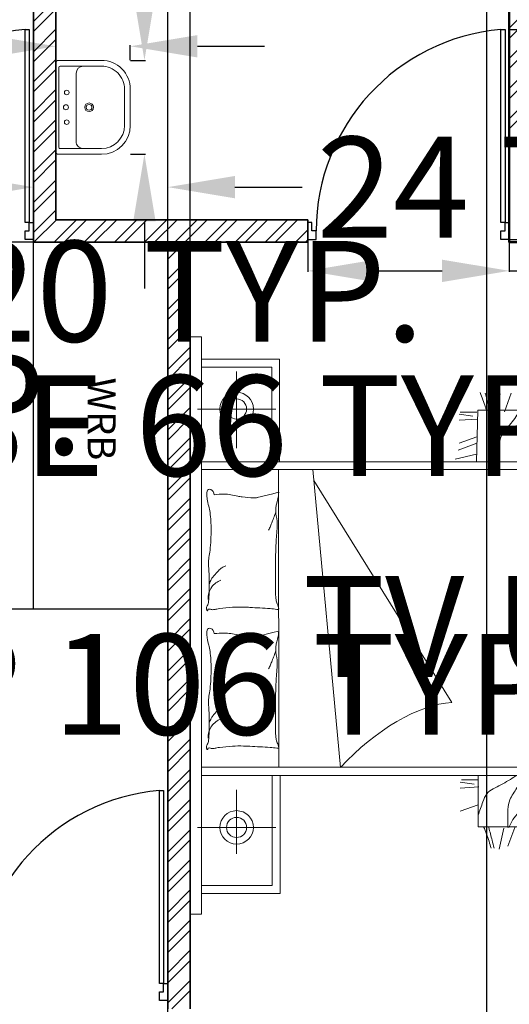
# Model space of a CAD drawing. Units: inches. Extents: x -90 to 536, y -553 to 299.
# Tile 23 of 27: x 207 to 294, y -2 to 174. Entities that reach past the tile are written whole.
import ezdxf

# ---------------------------------------------------------------- set-up
doc = ezdxf.new("R2010")
doc.units = ezdxf.units.IN
for name, color, linetype, lineweight in [('A-ANNO-DIMS', 2, 'Continuous', 18), ('A-ANNO-TEXT', 7, 'Continuous', 18), ('A-COLS', 7, 'Continuous', 50), ('A-DOOR', 4, 'Continuous', 25), ('A-FLOR-CASE', 2, 'Continuous', 25), ('A-FLOR-FIXT', 8, 'Continuous', 18), ('A-WALL-PATT', 252, 'Continuous', 13), ('Furniture', 2, 'Continuous', 18), ('Inner Wall', 5, 'Continuous', 35), ('Outer Wall', 1, 'Continuous', 50)]:
    doc.layers.add(name, color=color, linetype=linetype, lineweight=lineweight)
doc.styles.get("Standard").update_dxf_attribs({"font": 'arial.ttf'})
doc.dimstyles.get("Standard").update_dxf_attribs({"dimtxt": 18, "dimasz": 12, "dimexe": 0.18, "dimexo": 0.0625, "dimgap": 0.09, "dimtad": 0, "dimtih": 1, "dimtoh": 1, "dimdec": 0, "dimzin": 0, "dimdsep": 46, "dimlunit": 3, "dimtxsty": 'Standard', "dimcen": 0.09, "dimadec": 0, "dimazin": 0, "dimtfac": 1, "dimtdec": 0, "dimtofl": 0, "dimtmove": 0, "dimatfit": 3, "dimfxl": 1, "dimtolj": 1, "dimtzin": 0, "dimarcsym": 0})

# ---------------------------------------------------------------- blocks, each defined once
blk = doc.blocks.new('A$C57EA129C')
for p, q in [((0, 0.4428), (0, 0.1782)), ((0.016, 0.4589), (0.5631, 0.4589)), ((0.0356, 0.4321), (0.0356, 0.2896)), ((0.0445, 0.441), (0.5346, 0.441)), ((0.5435, 0.4321), (0.5435, 0.2896)), ((0.5791, 0.4428), (0.5791, 0.1782)), ((0.0802, 0.3341), (0.499, 0.3341)), ((0.0356, 0.2896), (0.0356, 0.1782)), ((0.5435, 0.2896), (0.5435, 0.1782)), ((0.1782, 0.0356), (0.4009, 0.0356)), ((0.1782, 0), (0.4009, 0))]:
    blk.add_line(p, q)
for centre, radius in [((0.1982, 0.392), 0.0143), ((0.2896, 0.3965), 0.0156), ((0.3809, 0.392), 0.0143), ((0.2896, 0.2545), 0.0267), ((0.2896, 0.2545), 0.0178)]:
    blk.add_circle(centre, radius)
for centre, radius, start, end in [((0.016, 0.4428), 0.016, 90, 180), ((0.0445, 0.4321), 0.00891, 90, 180), ((0.5346, 0.4321), 0.00891, 0, 90), ((0.5631, 0.4428), 0.016, 0, 90), ((0.0802, 0.2896), 0.0445, 90, 180), ((0.499, 0.2896), 0.0445, 0, 90), ((0.1782, 0.1782), 0.1782, 180, 270), ((0.1782, 0.1782), 0.1426, 180, 270), ((0.4009, 0.1782), 0.1782, 270, 0), ((0.4009, 0.1782), 0.1426, 270, 0)]:
    blk.add_arc(centre, radius, start, end)
blk = doc.blocks.new('A$C2B723114')
for p, q in [((0, 2.9047), (2.8274, 2.9047)), ((0, 2.8487), (0, 2.9047)), ((2.8274, 2.9047), (2.8274, 2.8487)), ((2.8274, 2.8487), (0, 2.8487)), ((0.1012, 2.4649), (0.1012, 2.849)), ((0.1396, 2.5033), (0.1396, 2.849)), ((0.4243, 2.8697), (0.4243, 2.4855)), ((0.6794, 0.7051), (0.6794, 2.8509)), ((0.7187, 0.7435), (0.7187, 2.8509)), ((2.1776, 2.8509), (2.1776, 0.7454)), ((2.216, 2.8509), (2.216, 0.707)), ((2.4742, 2.8697), (2.4742, 2.4855)), ((2.6798, 2.5052), (2.6798, 2.8509)), ((2.7182, 2.4668), (2.7182, 2.8509)), ((0.6087, 2.6776), (0.295, 2.6776)), ((2.6586, 2.6776), (2.2821, 2.6776)), ((1.3789, 2.4999), (1.3598, 2.5761)), ((2.0593, 2.4999), (2.0402, 2.5761)), ((0.6794, 2.4649), (0.1012, 2.4649)), ((0.6766, 2.5033), (0.1396, 2.5033)), ((0.7191, 2.47), (2.1778, 2.4719)), ((1.3858, 2.4723), (1.3789, 2.4999)), ((2.0662, 2.4723), (2.0593, 2.4999)), ((2.2188, 2.5052), (2.6798, 2.5052)), ((2.2188, 2.4668), (2.7182, 2.4668)), ((2.1771, 2.3036), (0.718, 2.1685)), ((1.0365, 1.6233), (2.1246, 2.2989)), ((2.2287, 1.6076), (2.2523, 1.5035)), ((2.2726, 1.593), (2.3061, 1.5007)), ((0.5047, 1.5819), (0.5353, 1.4945)), ((0.6174, 1.5819), (0.6232, 1.4916)), ((0.6467, 1.5819), (0.6369, 1.5137)), ((0.6571, 1.4945), (0.6571, 1.5765)), ((2.3067, 1.5881), (2.3373, 1.5007)), ((2.4194, 1.5881), (2.4251, 1.4979)), ((2.4487, 1.5881), (2.4389, 1.5199)), ((2.4591, 1.5007), (2.4591, 1.5828)), ((2.4685, 1.4964), (2.216, 1.5022)), ((2.4685, 1.4964), (2.4685, 0.0903)), ((0.4269, 0.0884), (0.4269, 1.4945)), ((0.4269, 1.4945), (0.6794, 1.4945)), ((2.4685, 1.4044), (2.5491, 1.3861)), ((0.3172, 1.3923), (0.4213, 1.3687)), ((2.4596, 1.3659), (2.552, 1.3324)), ((0.3318, 1.3485), (0.4241, 1.3149))]:
    blk.add_line(p, q)
for centre, radius in [((0.4243, 2.6776), 0.0821), ((2.4742, 2.6776), 0.0821), ((0.4243, 2.6776), 0.0493), ((2.4742, 2.6776), 0.0493)]:
    blk.add_circle(centre, radius)
for centre, radius, start, end in [((0.8078, 2.821), 0.00214, 160.436, 281.8931), ((0.8088, 2.8207), 0.00315, 111.7883, 160.436), ((0.8162, 2.8021), 0.0232, 94.3025, 111.7883), ((0.8091, 2.8151), 0.00394, 21.9904, 101.8931), ((0.8409, 2.7949), 0.0302, 158.579, 188.1335), ((0.7994, 2.8112), 0.0144, 338.579, 21.9904), ((0.8165, 2.7987), 0.0266, 59.3487, 94.3025), ((0.8554, 2.8643), 0.0497, 239.3487, 264.7408), ((0.9202, 3.5684), 0.7568, 264.7408, 268.0921), ((0.8679, 2.7254), 0.0915, 74.0648, 94.2159), ((0.8679, 2.7254), 0.0915, 53.9136, 74.0648), ((0.9409, 4.189), 1.3777, 268.0921, 270.5757), ((0.8679, 2.7254), 0.0915, 36.1766, 53.9136), ((0.86, 2.6097), 0.2158, 62.7604, 69.1397), ((0.9466, 3.6164), 0.8051, 270.5757, 274.8018), ((0.9263, 2.7386), 0.0708, 51.6114, 62.7604), ((1.0364, 2.548), 0.2671, 87.4614, 94.8018), ((1.042, 2.6745), 0.1405, 79.8101, 87.4614), ((1.1532, 3.2931), 0.488, 259.8101, 263.9133), ((1.204, 3.7695), 0.9671, 263.9133, 270), ((1.204, 3.4318), 0.6294, 270, 277.5469), ((1.2573, 3.0292), 0.2233, 277.5469, 285.744), ((1.3941, 2.5438), 0.281, 98.4372, 105.744), ((1.3747, 2.6748), 0.1486, 90, 98.4372), ((1.3713, 2.8186), 0.0315, 274.4002, 333.4195), ((1.3747, 2.74), 0.0833, 78.7276, 90), ((1.3886, 2.8099), 0.0121, 333.4195, 78.7276), ((1.4882, 2.821), 0.00214, 160.436, 281.8931), ((1.4892, 2.8207), 0.00315, 111.7883, 160.436), ((1.4966, 2.8021), 0.0232, 94.3025, 111.7883), ((1.4895, 2.8151), 0.00394, 21.9904, 101.8931), ((1.5213, 2.7949), 0.0302, 158.579, 188.1335), ((1.4798, 2.8112), 0.0144, 338.579, 21.9904), ((1.4969, 2.7987), 0.0266, 59.3487, 94.3025), ((1.5358, 2.8643), 0.0497, 239.3487, 264.7408), ((1.6006, 3.5684), 0.7568, 264.7408, 268.0921), ((1.5483, 2.7254), 0.0915, 74.0648, 94.2159), ((1.5483, 2.7254), 0.0915, 53.9136, 74.0648), ((1.6213, 4.189), 1.3777, 268.0921, 270.5757), ((1.5483, 2.7254), 0.0915, 36.1766, 53.9136), ((1.5404, 2.6097), 0.2158, 62.7604, 69.1397), ((1.627, 3.6164), 0.8051, 270.5757, 274.8018), ((1.6067, 2.7386), 0.0708, 51.6114, 62.7604), ((1.7168, 2.548), 0.2671, 87.4614, 94.8018), ((1.7224, 2.6745), 0.1405, 79.8101, 87.4614), ((1.8336, 3.2931), 0.488, 259.8101, 263.9133), ((1.8844, 3.7695), 0.9671, 263.9133, 270), ((1.8844, 3.4318), 0.6294, 270, 277.5469), ((1.9377, 3.0292), 0.2233, 277.5469, 285.744), ((2.0745, 2.5438), 0.281, 98.4372, 105.744), ((2.0551, 2.6748), 0.1486, 90, 98.4372), ((2.0517, 2.8186), 0.0315, 274.4002, 333.4195), ((2.0551, 2.74), 0.0833, 78.7276, 90), ((2.069, 2.8099), 0.0121, 333.4195, 78.7276), ((1.0356, 2.8227), 0.2268, 188.1335, 192.1095), ((0.635, 2.7368), 0.1829, 7.6809, 12.1095), ((-0.0181, 2.6487), 0.8418, 3.3687, 7.6809), ((0.8679, 2.7254), 0.0915, 18.4397, 36.1766), ((0.7461, 2.511), 0.3611, 46.1885, 51.6114), ((0.8523, 2.6218), 0.2076, 39.0349, 46.1885), ((0.9783, 2.7239), 0.0455, 28.3168, 39.0349), ((0.923, 2.7382), 0.4535, 0, 6.2324), ((1.716, 2.8227), 0.2268, 188.1335, 192.1095), ((1.3154, 2.7368), 0.1829, 7.6809, 12.1095), ((0.6623, 2.6487), 0.8418, 3.3687, 7.6809), ((1.5483, 2.7254), 0.0915, 18.4397, 36.1766), ((1.4265, 2.511), 0.3611, 46.1885, 51.6114), ((1.5327, 2.6218), 0.2076, 39.0349, 46.1885), ((1.6587, 2.7239), 0.0455, 28.3168, 39.0349), ((1.6034, 2.7382), 0.4535, 0, 6.2324), ((0.8558, 2.6579), 0.1846, 23.0028, 28.3168), ((0.5722, 2.8434), 0.8132, 347.8016, 350.3156), ((1.1884, 2.7382), 0.1881, 350.3156, 0), ((1.5362, 2.6579), 0.1846, 23.0028, 28.3168), ((1.2526, 2.8434), 0.8132, 347.8016, 350.3156), ((1.8688, 2.7382), 0.1881, 350.3156, 0), ((0.1976, 2.6614), 0.6258, 358.3669, 3.3687), ((1.6528, 2.6098), 0.2924, 167.8016, 171.9949), ((0.878, 2.6614), 0.6258, 358.3669, 3.3687), ((2.3332, 2.6098), 0.2924, 167.8016, 171.9949), ((-11.7321, 3.2823), 12.5718, 356.49514, 356.94504), ((-0.4351, 2.6794), 1.2587, 356.945, 358.3669), ((1.9648, 2.5659), 0.6074, 171.9949, 177.3351), ((-11.0517, 3.2823), 12.5718, 356.49514, 356.94504), ((0.2453, 2.6794), 1.2587, 356.945, 358.3669), ((2.6452, 2.5659), 0.6074, 171.9949, 177.3351), ((1.4204, 2.5912), 0.0624, 177.3351, 194.0452), ((2.1008, 2.5912), 0.0624, 177.3351, 194.0452), ((0.5206, 2.5319), 0.2961, 350.0016, 356.4951), ((1.4917, 3.1364), 0.681, 244.6889, 246.5156), ((1.4917, 3.1364), 0.681, 246.5156, 248.3423), ((1.201, 2.5319), 0.2961, 350.0016, 356.4951), ((2.1721, 3.1364), 0.681, 244.6889, 246.5156), ((2.1721, 3.1364), 0.681, 246.5156, 248.3423), ((0.8298, 2.4774), 0.0178, 170.0016, 196.6978), ((0.8139, 2.4726), 0.00122, 196.6978, 277.1204), ((0.8041, 2.5514), 0.0807, 277.1204, 286.2212), ((0.8068, 2.5419), 0.0707, 286.2212, 297.2841), ((0.8584, 2.4419), 0.0418, 102.869, 117.2841), ((0.879, 2.3515), 0.1345, 93.574, 102.869), ((0.9376, 1.4146), 1.0732, 90.2865, 93.574), ((0.9586, -2.7845), 5.2724, 89.0296, 90.2865), ((0.9954, -0.6123), 3.0999, 87.3904, 89.0296), ((1.0854, 1.364), 1.1216, 85.3824, 87.3904), ((1.28, 3.7729), 1.2952, 265.3824, 267.2509), ((1.228, 2.691), 0.2121, 267.2509, 281.5586), ((1.4917, 3.1364), 0.681, 248.3423, 250.572), ((1.4917, 3.1364), 0.681, 250.572, 252.8018), ((1.2975, 2.3514), 0.1345, 83.5659, 101.5586), ((1.3002, 2.3754), 0.1104, 72.6136, 83.5659), ((1.3965, 2.6828), 0.2118, 252.6136, 260.5159), ((1.4027, 2.7202), 0.2496, 260.5159, 265.9171), ((1.385, 2.4721), 0.000845, 265.9171, 14.0449), ((1.5102, 2.4774), 0.0178, 170.0016, 196.6978), ((1.4943, 2.4726), 0.00122, 196.6978, 277.1204), ((1.4845, 2.5514), 0.0807, 277.1204, 286.2212), ((1.4872, 2.5419), 0.0707, 286.2212, 297.2841), ((1.5388, 2.4419), 0.0418, 102.869, 117.2841), ((1.5594, 2.3515), 0.1345, 93.574, 102.869), ((1.618, 1.4146), 1.0732, 90.2865, 93.574), ((1.639, -2.7845), 5.2724, 89.0296, 90.2865), ((1.6758, -0.6123), 3.0999, 87.3904, 89.0296), ((1.7658, 1.364), 1.1216, 85.3824, 87.3904), ((1.9604, 3.7729), 1.2952, 265.3824, 267.2509), ((1.9084, 2.691), 0.2121, 267.2509, 281.5586), ((2.1721, 3.1364), 0.681, 248.3423, 250.572), ((2.1721, 3.1364), 0.681, 250.572, 252.8018), ((1.9779, 2.3514), 0.1345, 83.5659, 101.5586), ((1.9806, 2.3754), 0.1104, 72.6136, 83.5659), ((2.0769, 2.6828), 0.2118, 252.6136, 260.5159), ((2.0831, 2.7202), 0.2496, 260.5159, 265.9171), ((2.0654, 2.4721), 0.000845, 265.9171, 14.0449)]:
    blk.add_arc(centre, radius, start, end)
blk.add_ellipse((0.4962, 1.9132), major_axis=(0.4887, -0.4605), ratio=0.503305, start_param=0.491272, end_param=1.591113)
for points, knots in [([(0.427, 1.4678), (0.4036, 1.4582), (0.3693, 1.4441), (0.3335, 1.4344), (0.3221, 1.4313)], [0, 0, 0, 0, 98.452083, 144.639601, 144.639601, 144.639601, 144.639601]), ([(0.6768, 1.3104), (0.6615, 1.3339), (0.6315, 1.3797), (0.604, 1.4501), (0.5417, 1.4748), (0.5064, 1.4871), (0.4848, 1.4945)], [0, 0, 0, 0, 110.980521, 216.571322, 273.316778, 363.252298, 363.252298, 363.252298, 363.252298]), ([(2.5548, 1.4853), (2.5314, 1.4757), (2.5031, 1.4641), (2.4737, 1.4555), (2.4685, 1.454)], [0, 0, 0, 0, 98.452083, 119.481049, 119.481049, 119.481049, 119.481049]), ([(2.552, 1.4598), (2.5309, 1.4545), (2.5031, 1.4475), (2.4753, 1.4406), (2.4685, 1.4389)], [0, 0, 0, 0, 84.638756, 111.94623, 111.94623, 111.94623, 111.94623]), ([(0.4241, 1.4423), (0.4031, 1.437), (0.3691, 1.4284), (0.3351, 1.4199), (0.3221, 1.4167)], [0, 0, 0, 0, 84.638756, 136.955563, 136.955563, 136.955563, 136.955563]), ([(2.2145, 1.4211), (2.233, 1.4246), (2.2636, 1.4303), (2.2761, 1.3837), (2.3429, 1.3967), (2.3949, 1.3342), (2.4474, 1.3031), (2.4698, 1.2898)], [0, 0, 0, 0, 61.886907, 102.717887, 145.699352, 284.082577, 386.765171, 386.765171, 386.765171, 386.765171]), ([(0.6768, 1.286), (0.6567, 1.2911), (0.6145, 1.3017), (0.5543, 1.3533), (0.4816, 1.349), (0.4362, 1.3493), (0.4233, 1.3493)], [0, 0, 0, 0, 80.250278, 168.388677, 295.908361, 346.663112, 346.663112, 346.663112, 346.663112]), ([(0.4233, 1.3445), (0.4367, 1.3385), (0.464, 1.3264), (0.5129, 1.2848), (0.5456, 1.2161), (0.6131, 1.2349), (0.6142, 1.1913), (0.6642, 1.1806), (0.674, 1.144), (0.6817, 1.1154)], [0, 0, 0, 0, 56.745495, 115.23739, 254.956954, 286.678662, 337.828324, 366.201072, 468.500395, 468.500395, 468.500395, 468.500395])]:
    blk.add_open_spline(points, degree=3, knots=knots)
blk = doc.blocks.new('DOOR-36-A')
for points in [[(35.25, 37.5), (35.25, 3), (34.5, 3), (34.5, 37.5)], [(0, 0), (1.5, 0), (1.5, 1.5), (0.75, 1.5), (0.75, 3), (0, 3)], [(36, 0), (34.5, 0), (34.5, 1.5), (35.25, 1.5), (35.25, 3), (36, 3)]]:
    blk.add_lwpolyline(points, close=True)
blk.add_arc((37.64, 1.5), 36.14, 94.9791, 180)
blk = doc.blocks.new('COL-12X18')
blk.add_lwpolyline([(0, 18), (12, 18), (12, 0), (0, 0)], close=True)
blk = doc.blocks.new('WARDROBE')
blk.add_lwpolyline([(0, 65.56), (24, 65.56), (24, 0), (0, 0)], close=True)
blk = doc.blocks.new('*D19')
at = {"layer": 'A-ANNO-DIMS', "color": 0, "lineweight": -2, "transparency": 16777216}
for p, q in [((299.76, 172.45), (299.76, 184.45)), ((299.76, 184.45), (311.76, 184.45)), ((294.19, 172.45), (299.94, 172.45)), ((299.76, 146.95), (299.76, 160.45)), ((294.19, 134.95), (299.94, 134.95))]:
    blk.add_line(p, q, dxfattribs=at)
at = {"layer": 'A-ANNO-DIMS', "color": 0, "transparency": 16777216}
for points in [[(297.76, 160.45), (301.76, 160.45), (299.76, 172.45)], [(297.76, 146.95), (301.76, 146.95), (299.76, 134.95)]]:
    blk.add_solid(points, dxfattribs=at)
at = {"layer": 'Defpoints', "color": 0, "transparency": 16777216}
for p in [(294.13, 172.45), (299.76, 172.45), (294.13, 134.95)]:
    blk.add_point(p, dxfattribs=at)
at = {"layer": 'A-ANNO-DIMS', "color": 0, "transparency": 16777216, "insert": (408.3, 184.45), "char_height": 18, "attachment_point": 5}
blk.add_mtext('\\A1;DOOR A 38 TYP.', dxfattribs=at)
blk = doc.blocks.new('*D20')
at = {"layer": 'A-ANNO-DIMS', "color": 0, "lineweight": -2, "transparency": 16777216}
for p, q in [((258.13, 134.88), (258.13, 129.14)), ((294.13, 134.88), (294.13, 129.14)), ((270.13, 129.32), (282.13, 129.32)), ((294.13, 129.32), (306.13, 129.32))]:
    blk.add_line(p, q, dxfattribs=at)
at = {"layer": 'A-ANNO-DIMS', "color": 0, "transparency": 16777216}
for points in [[(270.13, 131.32), (270.13, 127.32), (258.13, 129.32)], [(282.13, 131.32), (282.13, 127.32), (294.13, 129.32)]]:
    blk.add_solid(points, dxfattribs=at)
at = {"layer": 'Defpoints', "color": 0, "transparency": 16777216}
for p in [(258.13, 134.95), (294.13, 134.95), (294.13, 129.32)]:
    blk.add_point(p, dxfattribs=at)
at = {"layer": 'A-ANNO-DIMS', "color": 0, "transparency": 16777216, "insert": (350.02, 129.32), "char_height": 18, "attachment_point": 5}
blk.add_mtext('\\A1;36 TYP.', dxfattribs=at)
blk = doc.blocks.new('*D25')
at = {"layer": 'A-ANNO-DIMS', "color": 0, "lineweight": -2, "transparency": 16777216}
for p, q in [((228.95, 178.94), (228.95, 190.94)), ((228.95, 190.94), (240.95, 190.94)), ((226.49, 166.94), (229.13, 166.94)), ((226.49, 150.15), (229.13, 150.15)), ((228.95, 138.15), (228.95, 126.15))]:
    blk.add_line(p, q, dxfattribs=at)
at = {"layer": 'A-ANNO-DIMS', "color": 0, "transparency": 16777216}
for points in [[(226.95, 178.94), (230.95, 178.94), (228.95, 166.94)], [(226.95, 138.15), (230.95, 138.15), (228.95, 150.15)]]:
    blk.add_solid(points, dxfattribs=at)
at = {"layer": 'Defpoints', "color": 0, "transparency": 16777216}
for p in [(226.43, 166.94), (228.95, 166.94), (226.43, 150.15)]:
    blk.add_point(p, dxfattribs=at)
at = {"layer": 'A-ANNO-DIMS', "color": 0, "transparency": 16777216, "insert": (325.67, 190.94), "char_height": 18, "attachment_point": 5}
blk.add_mtext('\\A1;BASIN 17 TYP.', dxfattribs=at)
blk = doc.blocks.new('*D26')
at = {"layer": 'A-ANNO-DIMS', "color": 0, "lineweight": -2, "transparency": 16777216}
for p, q in [((201.13, 169.45), (189.13, 169.45)), ((213.13, 167), (213.13, 169.63)), ((226.43, 167), (226.43, 169.63)), ((238.43, 169.45), (250.43, 169.45))]:
    blk.add_line(p, q, dxfattribs=at)
at = {"layer": 'A-ANNO-DIMS', "color": 0, "transparency": 16777216}
for points in [[(201.13, 171.45), (201.13, 167.45), (213.13, 169.45)], [(238.43, 171.45), (238.43, 167.45), (226.43, 169.45)]]:
    blk.add_solid(points, dxfattribs=at)
at = {"layer": 'Defpoints', "color": 0, "transparency": 16777216}
for p in [(213.13, 169.45), (213.13, 166.94), (226.43, 166.94)]:
    blk.add_point(p, dxfattribs=at)
at = {"layer": 'A-ANNO-DIMS', "color": 0, "transparency": 16777216, "insert": (146.08, 169.45), "char_height": 18, "attachment_point": 5}
blk.add_mtext('\\A1;13 TYP.', dxfattribs=at)
blk = doc.blocks.new('*D29')
at = {"layer": 'A-ANNO-DIMS', "color": 0, "lineweight": -2, "transparency": 16777216}
for p, q in [((357.07, 98.65), (347.09, 98.65)), ((347.27, 86.65), (347.27, 75.05)), ((347.27, 44.88), (347.27, 56.48)), ((357.07, 32.88), (347.09, 32.88))]:
    blk.add_line(p, q, dxfattribs=at)
at = {"layer": 'A-ANNO-DIMS', "color": 0, "transparency": 16777216}
for points in [[(345.27, 86.65), (349.27, 86.65), (347.27, 98.65)], [(345.27, 44.88), (349.27, 44.88), (347.27, 32.88)]]:
    blk.add_solid(points, dxfattribs=at)
at = {"layer": 'Defpoints', "color": 0, "transparency": 16777216}
for p in [(347.27, 98.65), (357.13, 98.65), (357.13, 32.88)]:
    blk.add_point(p, dxfattribs=at)
at = {"layer": 'A-ANNO-DIMS', "color": 0, "transparency": 16777216, "insert": (347.27, 65.76), "char_height": 18, "attachment_point": 5}
blk.add_mtext('\\A1;TV UNIT 66 TYP.', dxfattribs=at)
blk = doc.blocks.new('*D31')
at = {"layer": 'A-ANNO-DIMS', "color": 0, "lineweight": -2, "transparency": 16777216}
for p, q in [((90.45, 119.36), (100.65, 125.67)), ((100.65, 125.67), (112.65, 125.67)), ((78.67, 115.59), (80.34, 112.89)), ((61.33, 104.86), (63, 102.15)), ((52.7, 95.99), (42.5, 89.68))]:
    blk.add_line(p, q, dxfattribs=at)
at = {"layer": 'A-ANNO-DIMS', "color": 0, "transparency": 16777216}
for points in [[(89.4, 121.06), (91.5, 117.65), (80.24, 113.04)], [(51.65, 97.69), (53.76, 94.29), (62.91, 102.31)]]:
    blk.add_solid(points, dxfattribs=at)
at = {"layer": 'Defpoints', "color": 0, "transparency": 16777216}
for p in [(78.63, 115.64), (80.24, 113.04), (61.3, 104.91)]:
    blk.add_point(p, dxfattribs=at)
at = {"layer": 'A-ANNO-DIMS', "color": 0, "transparency": 16777216, "insert": (199.06, 125.67), "char_height": 18, "attachment_point": 5}
blk.add_mtext('\\A1;CHAIR 20 TYP.', dxfattribs=at)
blk = doc.blocks.new('*D33')
at = {"layer": 'A-ANNO-DIMS', "color": 0, "lineweight": -2, "transparency": 16777216}
for p, q in [((173.76, 108.4), (189.77, 108.4)), ((189.59, 96.4), (189.59, 64.83)), ((189.59, 14.45), (189.59, 46.02)), ((173.76, 2.45), (189.77, 2.45))]:
    blk.add_line(p, q, dxfattribs=at)
at = {"layer": 'A-ANNO-DIMS', "color": 0, "transparency": 16777216}
for points in [[(187.59, 96.4), (191.59, 96.4), (189.59, 108.4)], [(187.59, 14.45), (191.59, 14.45), (189.59, 2.45)]]:
    blk.add_solid(points, dxfattribs=at)
at = {"layer": 'Defpoints', "color": 0, "transparency": 16777216}
for p in [(173.7, 108.4), (173.7, 2.45), (189.59, 2.45)]:
    blk.add_point(p, dxfattribs=at)
at = {"layer": 'A-ANNO-DIMS', "color": 0, "transparency": 16777216, "insert": (189.59, 55.42), "char_height": 18, "attachment_point": 5}
blk.add_mtext('\\A1;BED GROUP 106 TYP.', dxfattribs=at)
blk = doc.blocks.new('*D37')
at = {"layer": 'A-ANNO-DIMS', "color": 0, "lineweight": -2, "transparency": 16777216}
for p, q in [((35.09, 103.75), (35.09, 105.68)), ((47.13, 103.75), (47.13, 105.68)), ((23.09, 105.5), (11.09, 105.5)), ((59.13, 105.5), (71.13, 105.5))]:
    blk.add_line(p, q, dxfattribs=at)
at = {"layer": 'A-ANNO-DIMS', "color": 0, "transparency": 16777216}
for points in [[(23.09, 107.5), (23.09, 103.5), (35.09, 105.5)], [(59.13, 107.5), (59.13, 103.5), (47.13, 105.5)]]:
    blk.add_solid(points, dxfattribs=at)
at = {"layer": 'Defpoints', "color": 0, "transparency": 16777216}
for p in [(47.13, 105.5), (35.09, 103.69), (47.13, 103.69)]:
    blk.add_point(p, dxfattribs=at)
at = {"layer": 'A-ANNO-DIMS', "color": 0, "transparency": 16777216, "insert": (147.42, 105.5), "char_height": 18, "attachment_point": 5}
blk.add_mtext('\\A1;PIER 12 TYP.', dxfattribs=at)
blk = doc.blocks.new('*D39')
at = {"layer": 'A-ANNO-DIMS', "color": 0, "lineweight": -2, "transparency": 16777216}
for p, q in [((209.07, 134.45), (199.12, 134.45)), ((199.3, 122.45), (199.3, 111.07)), ((199.3, 80.89), (199.3, 92.26)), ((209.07, 68.89), (199.12, 68.89))]:
    blk.add_line(p, q, dxfattribs=at)
at = {"layer": 'A-ANNO-DIMS', "color": 0, "transparency": 16777216}
for points in [[(197.3, 122.45), (201.3, 122.45), (199.3, 134.45)], [(197.3, 80.89), (201.3, 80.89), (199.3, 68.89)]]:
    blk.add_solid(points, dxfattribs=at)
at = {"layer": 'Defpoints', "color": 0, "transparency": 16777216}
for p in [(199.3, 134.45), (209.13, 134.45), (209.13, 68.89)]:
    blk.add_point(p, dxfattribs=at)
at = {"layer": 'A-ANNO-DIMS', "color": 0, "transparency": 16777216, "insert": (199.3, 101.67), "char_height": 18, "attachment_point": 5}
blk.add_mtext('\\A1;WARDROBE 66 TYP.', dxfattribs=at)
blk = doc.blocks.new('*D40')
at = {"layer": 'A-ANNO-DIMS', "color": 0, "lineweight": -2, "transparency": 16777216}
for p, q in [((209.13, 134.51), (209.13, 144.46)), ((233.13, 134.51), (233.13, 144.46)), ((197.13, 144.28), (185.13, 144.28)), ((245.13, 144.28), (257.13, 144.28))]:
    blk.add_line(p, q, dxfattribs=at)
at = {"layer": 'A-ANNO-DIMS', "color": 0, "transparency": 16777216}
for points in [[(197.13, 146.28), (197.13, 142.28), (209.13, 144.28)], [(245.13, 146.28), (245.13, 142.28), (233.13, 144.28)]]:
    blk.add_solid(points, dxfattribs=at)
at = {"layer": 'Defpoints', "color": 0, "transparency": 16777216}
for p in [(233.13, 144.28), (209.13, 134.45), (233.13, 134.45)]:
    blk.add_point(p, dxfattribs=at)
at = {"layer": 'A-ANNO-DIMS', "color": 0, "transparency": 16777216, "insert": (301.18, 144.28), "char_height": 18, "attachment_point": 5}
blk.add_mtext('\\A1;24 TYP.', dxfattribs=at)
blk = doc.blocks.new('*D53')
at = {"layer": 'A-ANNO-DIMS', "color": 0, "lineweight": -2, "transparency": 16777216}
for p, q in [((35.09, 103.75), (35.09, 287.38)), ((47.09, 287.2), (183.7, 287.2)), ((395.13, 287.2), (258.52, 287.2)), ((407.13, -63.49), (407.13, 287.38))]:
    blk.add_line(p, q, dxfattribs=at)
at = {"layer": 'A-ANNO-DIMS', "color": 0, "transparency": 16777216}
for points in [[(47.09, 289.2), (47.09, 285.2), (35.09, 287.2)], [(395.13, 289.2), (395.13, 285.2), (407.13, 287.2)]]:
    blk.add_solid(points, dxfattribs=at)
at = {"layer": 'Defpoints', "color": 0, "transparency": 16777216}
for p in [(407.13, 287.2), (35.09, 103.69), (407.13, -63.55)]:
    blk.add_point(p, dxfattribs=at)
at = {"layer": 'A-ANNO-DIMS', "color": 0, "transparency": 16777216, "insert": (221.11, 287.2), "char_height": 18, "attachment_point": 5}
blk.add_mtext('\\A1;372.04', dxfattribs=at)
blk = doc.blocks.new('*D58')
at = {"layer": 'A-ANNO-DIMS', "color": 0, "lineweight": -2, "transparency": 16777216}
for p, q in [((290.13, -71.49), (290.13, 287.38)), ((302.13, 287.2), (308.6, 287.2)), ((341.13, 287.2), (334.66, 287.2)), ((353.13, -71.49), (353.13, 287.38))]:
    blk.add_line(p, q, dxfattribs=at)
at = {"layer": 'A-ANNO-DIMS', "color": 0, "transparency": 16777216}
for points in [[(302.13, 289.2), (302.13, 285.2), (290.13, 287.2)], [(341.13, 289.2), (341.13, 285.2), (353.13, 287.2)]]:
    blk.add_solid(points, dxfattribs=at)
at = {"layer": 'Defpoints', "color": 0, "transparency": 16777216}
for p in [(353.13, 287.2), (290.13, -71.55), (353.13, -71.55)]:
    blk.add_point(p, dxfattribs=at)
at = {"layer": 'A-ANNO-DIMS', "color": 0, "transparency": 16777216, "insert": (321.63, 287.2), "char_height": 18, "attachment_point": 5}
blk.add_mtext('\\A1;63', dxfattribs=at)
blk = doc.blocks.new('*D62')
at = {"layer": 'A-ANNO-DIMS', "color": 0, "lineweight": -2, "transparency": 16777216}
for p, q in [((233.13, -71.49), (233.13, 287.38)), ((245.13, 287.2), (248.65, 287.2)), ((278.13, 287.2), (274.61, 287.2)), ((290.13, -71.49), (290.13, 287.38))]:
    blk.add_line(p, q, dxfattribs=at)
at = {"layer": 'A-ANNO-DIMS', "color": 0, "transparency": 16777216}
for points in [[(245.13, 289.2), (245.13, 285.2), (233.13, 287.2)], [(278.13, 289.2), (278.13, 285.2), (290.13, 287.2)]]:
    blk.add_solid(points, dxfattribs=at)
at = {"layer": 'Defpoints', "color": 0, "transparency": 16777216}
for p in [(290.13, 287.2), (233.13, -71.55), (290.13, -71.55)]:
    blk.add_point(p, dxfattribs=at)
at = {"layer": 'A-ANNO-DIMS', "color": 0, "transparency": 16777216, "insert": (261.63, 287.2), "char_height": 18, "attachment_point": 5}
blk.add_mtext('\\A1;57', dxfattribs=at)
blk = doc.blocks.new('*D65')
at = {"layer": 'A-ANNO-DIMS', "color": 0, "lineweight": -2, "transparency": 16777216}
for p, q in [((221.13, 287.2), (209.13, 287.2)), ((233.13, 134.51), (233.13, 287.38)), ((237.13, 134.51), (237.13, 287.38)), ((249.13, 287.2), (261.13, 287.2))]:
    blk.add_line(p, q, dxfattribs=at)
at = {"layer": 'A-ANNO-DIMS', "color": 0, "transparency": 16777216}
for points in [[(221.13, 289.2), (221.13, 285.2), (233.13, 287.2)], [(249.13, 289.2), (249.13, 285.2), (237.13, 287.2)]]:
    blk.add_solid(points, dxfattribs=at)
at = {"layer": 'Defpoints', "color": 0, "transparency": 16777216}
for p in [(237.13, 287.2), (233.13, 134.45), (237.13, 134.45)]:
    blk.add_point(p, dxfattribs=at)
at = {"layer": 'A-ANNO-DIMS', "color": 0, "transparency": 16777216, "insert": (267.45, 287.2), "char_height": 18, "attachment_point": 5}
blk.add_mtext('\\A1;4', dxfattribs=at)

msp = doc.modelspace()

# ---------------------------------------------------------------- hatches: boundary and pattern name
at = {"layer": 'A-WALL-PATT'}
h = msp.add_hatch(dxfattribs=at)
h.set_pattern_fill('ANSI32', color=256, scale=0.4)
h.set_pattern_definition([(45, (-88.8105, -603.6155), (-2.694077, 2.694077), []), (45, (-87.0145, -603.6155), (-2.694077, 2.694077), [])])
h.paths.add_polyline_path([(285.1317, 246.4462), (131.1317, 246.4462), (131.1317, 237.4462), (285.1317, 237.4462)])
h.paths.add_polyline_path([(122.1317, 237.4462), (113.1317, 237.4462), (113.1317, 152.4462), (122.1317, 152.4462), (122.1317, 166.4704)])
h.paths.add_polyline_path([(303.1317, 237.4462), (294.1317, 237.4462), (294.1317, 152.4462), (303.1317, 152.4462)])
h.paths.add_polyline_path([(47.1317, 91.9277), (38.1317, 91.9277), (38.1317, -6.5538), (77.1317, -6.5538), (77.1317, 2.4462), (70.5655, 2.4462), (47.1317, 2.4462)])
h.paths.add_polyline_path([(83.052, -61.5538), (47.1317, -61.5538), (47.1317, -24.5538), (38.1317, -24.5538), (38.1317, -70.5538), (74.052, -70.5538), (74.052, -223.5538), (38.1317, -223.5538), (38.1317, -503.5538), (92.1317, -503.5538), (92.1317, -437.5538), (191.1317, -437.5538), (191.1317, -428.5538), (83.1317, -428.5538), (83.1317, -494.5538), (47.1317, -494.5538), (47.1317, -232.5538), (83.052, -232.5538), (83.052, -70.5538)])
h.paths.add_polyline_path([(407.1317, -63.5538), (381.1317, -63.5538), (381.1317, 91.9277), (372.1317, 91.9277), (372.1317, 32.8805), (372.1317, -63.5538), (306.5745, -63.5538), (237.1317, -63.5538), (237.1317, -38.5538), (233.1317, -38.5538), (233.1317, -71.5538), (398.1317, -71.5538), (398.1317, -152.5538), (233.1317, -152.5538), (233.1317, -161.5538), (398.1317, -161.5538), (398.1317, -368.5538), (233.1317, -368.5538), (233.1317, -377.5538), (407.1317, -377.5538), (407.1317, -161.5538)])
h.paths.add_polyline_path([(261.1317, -422.5538), (252.1317, -422.5538), (252.1317, -428.5538), (233.1317, -428.5538), (233.1317, -437.5538), (261.1317, -437.5538)])
h.paths.add_polyline_path([(191.1317, -368.5538), (180.1317, -368.5538), (180.1317, -335.5538), (131.5919, -335.5538), (131.5919, -344.5538), (171.1317, -344.5538), (171.1317, -392.5538), (180.1317, -392.5538), (180.1317, -377.5538), (191.1317, -377.5538)], flags=17)
h.paths.add_polyline_path([(180.1317, -223.5538), (152.1317, -223.5538), (152.1317, -227.5538), (176.1317, -227.5538), (176.1317, -335.5538), (180.1317, -335.5538)], flags=17)
h.paths.add_polyline_path([(131.5919, -335.5538), (83.1317, -335.5538), (83.1317, -339.5538), (83.1317, -392.5538), (87.1317, -392.5538), (87.1317, -339.5538), (131.5919, -339.5538)], flags=17)
h.paths.add_polyline_path([(197.1317, 2.4462), (77.1317, 2.4462), (77.1317, -1.5538), (113.1317, -1.5538), (113.1317, -71.5538), (181.1317, -71.5538), (181.1317, -67.5538), (117.1317, -67.5538), (117.1317, -1.5538), (177.1317, -1.5538), (177.1317, -37.5538), (181.1317, -37.5538), (181.1317, -1.5538), (197.1317, -1.5538)])
h.paths.add_polyline_path([(173.1317, 138.4462), (122.1317, 138.4462), (122.1317, 134.4462), (173.1317, 134.4462)])
h.paths.add_polyline_path([(213.1317, 237.4462), (209.1317, 237.4462), (209.1317, 134.4462), (233.1317, 134.4462), (233.1317, 68.8889), (233.1317, -2.5538), (237.1317, -2.5538), (237.1317, 134.4462), (258.1317, 134.4462), (258.1317, 138.4462), (213.1317, 138.4462)])

# ---------------------------------------------------------------- linework, layer by layer
at = {"layer": 'Inner Wall'}
for p, q in [((209.1317, 237.4462), (209.1317, 134.4462)), ((213.1317, 237.4462), (213.1317, 138.4462)), ((258.1317, 138.4462), (213.1317, 138.4462)), ((258.1317, 138.4462), (258.1317, 134.4462)), ((233.1317, 134.4462), (209.1317, 134.4462)), ((233.1317, 134.4462), (233.1317, -2.5538)), ((258.1317, 134.4462), (237.1317, 134.4462)), ((237.1317, 134.4462), (237.1317, -2.5538))]:
    msp.add_line(p, q, dxfattribs=at)
at = {"layer": 'Outer Wall'}
msp.add_line((294.1317, 237.4462), (294.1317, 134.4462), dxfattribs=at)

# ---------------------------------------------------------------- block references
at = {"layer": 'A-COLS'}
msp.add_blockref('COL-12X18', (294.1317, 134.4462), dxfattribs=at)
at = {"layer": 'A-DOOR'}
for p in [(173.1317, 134.9462), (258.1317, 134.9462), (197.1317, -1.0538)]:
    msp.add_blockref('DOOR-36-A', p, dxfattribs=at)
at = {"layer": 'A-FLOR-CASE'}
msp.add_blockref('WARDROBE', (209.1317, 68.8889), dxfattribs=at)
at = {"layer": 'A-FLOR-FIXT', "xscale": 28.98333223671166, "yscale": 28.98333223671166, "zscale": 28.98333223671166, "rotation": 89.99999999999999}
msp.add_blockref('A$C57EA129C', (226.4312, 150.1495), dxfattribs=at)
at = {"layer": 'Furniture', "xscale": 36.47664764473289, "yscale": 36.47664764473289, "zscale": 36.47664764473289, "rotation": 89.99999999999999}
msp.add_blockref('A$C2B723114', (343.0864, 14.3799), dxfattribs=at)

# ---------------------------------------------------------------- texts
at = {"layer": 'A-ANNO-TEXT', "insert": (223.831, 85.2373), "char_height": 5, "attachment_point": 3, "rotation": 270}
msp.add_mtext_dynamic_manual_height_columns('\\pxqc;{\\fTimes New Roman|b0|i0|c0|p18;WRB}', width=35.23368, gutter_width=12.5, heights=[0], dxfattribs=at)

# ---------------------------------------------------------------- dimensions: what is measured, and where the dimension line sits
at = {"layer": 'A-ANNO-DIMS'}
for base, p1, p2, override, picture, middle in [((407.1317, 287.2012), (35.0873, 103.6916), (407.1317, -63.5538), {"dimdec": 2, "dimlfac": 1, "dimrnd": 0, "dimzin": 0, "dimdsep": 46, "dimlunit": 2}, '*D53', (221.1095, 287.2012)), ((237.1317, 287.2012), (233.1317, 134.4462), (237.1317, 134.4462), {"dimdec": 0, "dimlfac": 1, "dimrnd": 0, "dimzin": 0, "dimdsep": 46, "dimlunit": 2}, '*D65', (267.4468, 287.2012)), ((290.1317, 287.2012), (233.1317, -71.5538), (290.1317, -71.5538), {"dimdec": 0, "dimlfac": 1, "dimrnd": 0, "dimzin": 0, "dimdsep": 46, "dimlunit": 2}, '*D62', (261.6317, 287.2012)), ((353.1317, 287.2012), (290.1317, -71.5538), (353.1317, -71.5538), {"dimdec": 0, "dimlfac": 1, "dimrnd": 0, "dimzin": 0, "dimdsep": 46, "dimlunit": 2}, '*D58', (321.6317, 287.2012))]:
    dim = msp.add_linear_dim(base=base, p1=p1, p2=p2, dimstyle='Standard', override=override, dxfattribs=at)
    dim.commit()
    dim.dimension.update_dxf_attribs({"geometry": picture, "text_midpoint": middle})
for base, p1, p2, angle, text, picture, middle in [((299.7567404714, 172.4462174295), (294.1317404714, 134.9462174295), (294.1317404714, 172.4462174295), 90, 'DOOR A <> TYP.', '*D19', (408.2989914946, 184.4462174295)), ((228.949, 166.9352), (226.4312, 150.1495), (226.4312, 166.9352), 90, 'BASIN <> TYP.', '*D25', (325.6734, 190.9352)), ((213.1317, 169.4531), (226.4312, 166.9352), (213.1317, 166.9352), 180, '<> TYP.', '*D26', (146.0799, 169.4531)), ((80.2442, 113.0397), (61.2964, 104.9085), (78.6344, 115.6404), 31.756702, 'CHAIR <> TYP.', '*D31', (199.0577, 125.6712)), ((199.2981, 134.4462), (209.1317, 68.8889), (209.1317, 134.4462), 90, 'WARDROBE <> TYP.', '*D39', (199.2981, 101.6676)), ((347.2664, 98.6495), (357.1317, 32.8805), (357.1317, 98.6495), 90, 'TV UNIT <> TYP.', '*D29', (347.2664, 65.765)), ((189.5912, 2.4462), (173.698, 108.4009), (173.698, 2.4462), 270, 'BED GROUP <> TYP.', '*D33', (189.5912, 55.4235))]:
    dim = msp.add_linear_dim(base=base, p1=p1, p2=p2, angle=angle, text=text, dimstyle='Standard', override={"dimdec": 0, "dimlfac": 1, "dimrnd": 0, "dimzin": 0, "dimdsep": 46, "dimlunit": 2}, dxfattribs=at)
    dim.commit()
    dim.dimension.update_dxf_attribs({"geometry": picture, "text_midpoint": middle})
for base, p1, p2, text, picture, middle in [((233.1317, 144.2798), (209.1317, 134.4462), (233.1317, 134.4462), '<> TYP.', '*D40', (301.1842, 144.2798)), ((294.1317, 129.3212), (258.1317, 134.9462), (294.1317, 134.9462), '<> TYP.', '*D20', (350.0246, 129.3212)), ((47.1317, 105.4983), (35.0873, 103.6916), (47.1317, 103.6916), 'PIER <> TYP.', '*D37', (147.4209, 105.4983))]:
    dim = msp.add_linear_dim(base=base, p1=p1, p2=p2, text=text, dimstyle='Standard', override={"dimdec": 0, "dimlfac": 1, "dimrnd": 0, "dimzin": 0, "dimdsep": 46, "dimlunit": 2}, dxfattribs=at)
    dim.commit()
    dim.dimension.update_dxf_attribs({"geometry": picture, "text_midpoint": middle})

doc.saveas('drawing.dxf')
